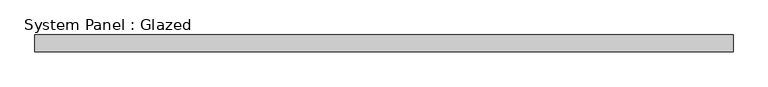
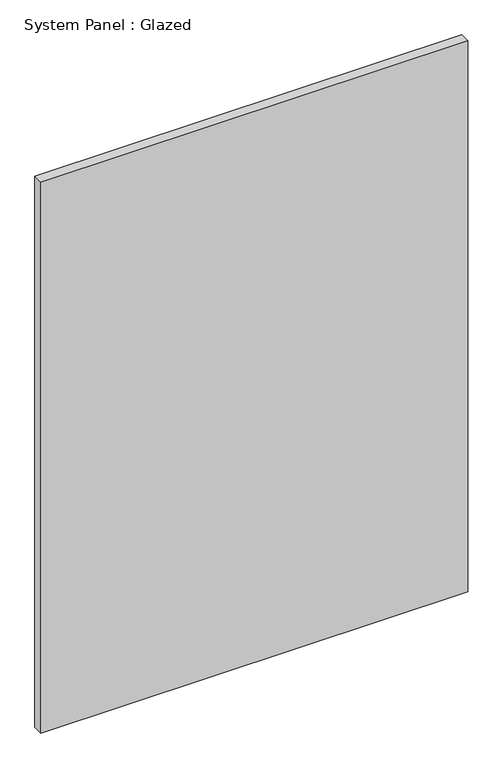
"""IFC4 building model written with IfcOpenShell, lengths in millimetres: plate geometry, System Panel : Glazed."""

from ifc_helpers import new_model, si_unit, origin, origin_with_axes, place, context, project, spatial, polyline, outline, extrude, source, transform, mapped, element, save


def system_panel_glazed_36abd0f2(model_context):
    return source(origin(), model_context, "Body", "SweptSolid", [
        extrude(outline(polyline([(523.875, 19.05), (-523.875, 19.05), (-523.875, 44.45), (523.875, 44.45), (523.875, 19.05)])), origin_with_axes(), (0.0, 0.0, 1.0), 1428.75),
    ])


if __name__ == "__main__":
    model = new_model("IFC4")
    model_context = context("Model", 3, world=origin())
    ifc_project = project(units=[si_unit("LENGTHUNIT", "METRE", prefix="MILLI")], contexts=[model_context])
    site = spatial("IfcSite", under=ifc_project)
    building = spatial("IfcBuilding", under=site)
    placement = place(None, origin())
    system_panel_glazed_shape = system_panel_glazed_36abd0f2(model_context)
    element("IfcPlate", 1, ObjectType="System Panel : Glazed", at=placement, inside=building, context=model_context, shape_type="MappedRepresentation", body=[
        mapped(system_panel_glazed_shape, transform((0.0, 0.0, 0.0), x_axis=(1.0, 0.0, 0.0), y_axis=(0.0, 1.0, 0.0), z_axis=(0.0, 0.0, 1.0))),
    ])
    save(model, "model.ifc")

# Revit data of these elements
# Type "System Panel : Glazed"
#   Construction Type Id = "GSP4R"
#   Analytic Construction = "1/8 in Pilkington single glazing"
#   Visual Light Transmittance = 0.9
#   Solar Heat Gain Coefficient = 0.86
#   Heat Transfer Coefficient (U) = 1.18115 BTU/(h·ft²·°F)
#   Define Thermal Properties by = 1
# Element 1 (IfcPlate, "System Panel : Glazed")
#   Materials on its faces: "Glass"
# Materials
#   "Glass": class "Glass", colour RGB 0 128 192, transparency 0.75, Description = "Soda Lime Glass", Cost = 0
